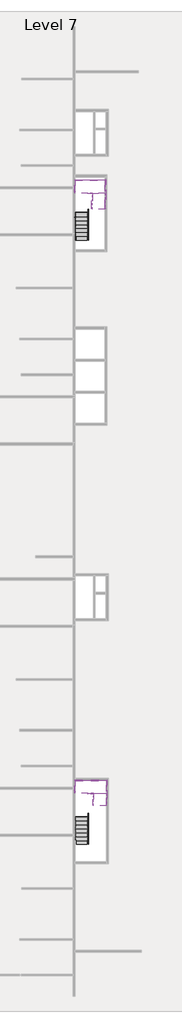
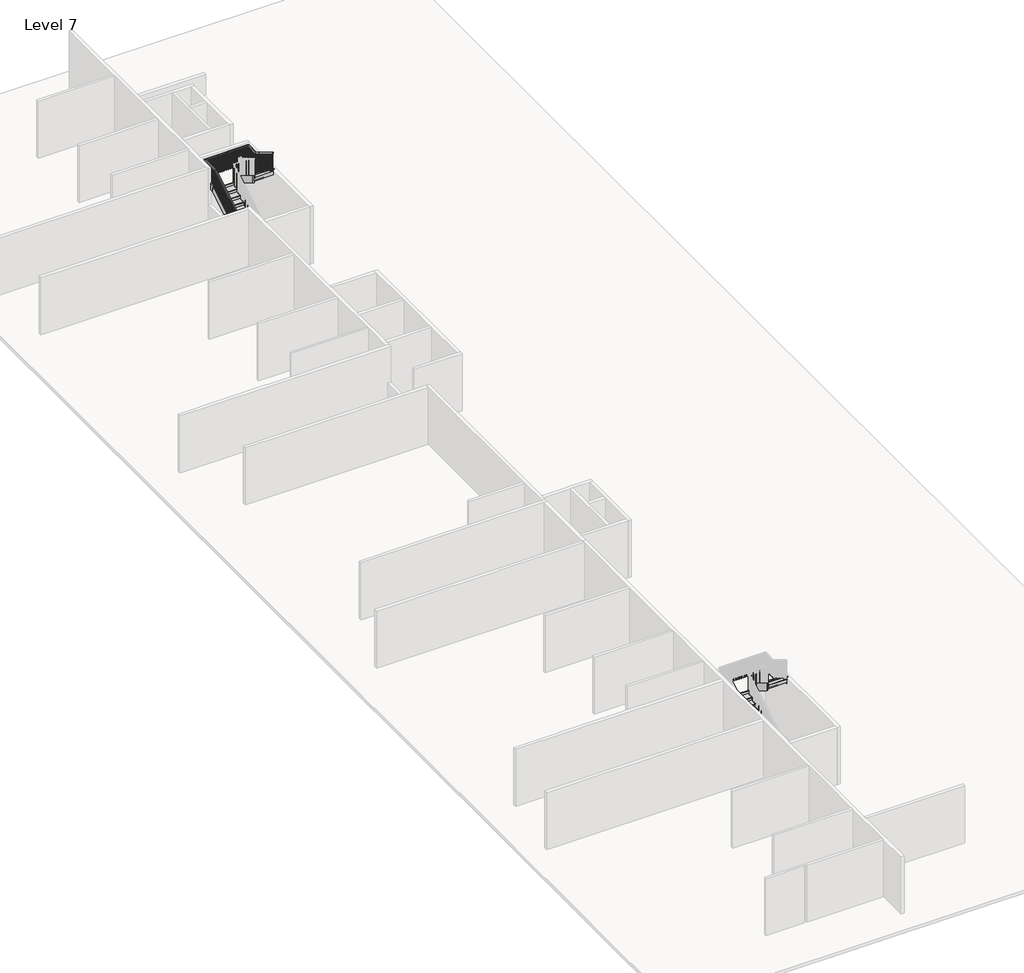
# One storey, part 8 of 8: 16 members, 4 stair flights, 2 slabs, 1 railing.
"""IFC4 building model written with IfcOpenShell, lengths in millimetres."""

from ifc_helpers import new_model, si_unit, frame, origin, place, context, project, spatial, polyline, outline, extrude, faceted_brep, transform, mapped, element, save
from components import non_monolithic_landing_71f31ac1, non_monolithic_landing_55824b8c, stair_flight_36526160, stair_flight_c8914c85, stair_flight_f72f160c, stair_flight_d5778488

model = new_model("IFC4")

# Units and contexts
model_context = context("Model", 3, world=origin())
ifc_project = project(units=[si_unit("LENGTHUNIT", "METRE", prefix="MILLI")], contexts=[model_context])

# Site, building, storey
site = spatial("IfcSite", under=ifc_project)
building = spatial("IfcBuilding", under=site)
storey = spatial("IfcBuildingStorey", under=building, Name="Level 7", Elevation=43522.6172466)

# Members
placement = place(None, origin())
element("IfcMember", 1, ObjectType="Stringer - 2\" Width", at=placement, inside=storey, context=model_context, shape_type="SweptSolid", body=[
    extrude(outline(polyline([(-23154.3851539, 43522.6172466), (-23154.3851539, 43734.7317586), (-19467.0440987, 45969.4839133), (-19381.8896422, 45664.6839133), (-22916.2996422, 43522.6172466), (-23154.3851539, 43522.6172466)])), frame((-3668.2415084, 0.0, 0.0), z_axis=(1.0, 0.0, 0.0), x_axis=(0.0, 1.0, 0.0)), (0.0, 0.0, 1.0), 50.8),
])
element("IfcMember", 2, ObjectType="Stringer - 2\" Width", at=placement, inside=storey, context=model_context, shape_type="SweptSolid", body=[
    extrude(outline(polyline([(-23154.3851539, 43522.6172466), (-23154.3851539, 43734.7317586), (-19572.9851539, 45905.2772131), (-19572.9851539, 45548.8684516), (-22916.2996422, 43522.6172466), (-23154.3851539, 43522.6172466)])), frame((-2703.0415084, 0.0, 0.0), z_axis=(1.0, 0.0, 0.0), x_axis=(0.0, 1.0, 0.0)), (0.0, 0.0, 1.0), 50.8),
])
element("IfcMember", 3, ObjectType="Stringer - 2\" Width", at=placement, inside=storey, context=model_context, shape_type="SweptSolid", body=[
    extrude(outline(polyline([(-19297.9262092, 45969.4839133), (-19383.0806657, 45664.6839133), (-20360.3851539, 46256.9896637), (-20360.3851539, 46613.3984252), (-19297.9262092, 45969.4839133)])), frame((-1382.2415084, 0.0, 0.0), z_axis=(1.0, 0.0, 0.0), x_axis=(0.0, 1.0, 0.0)), (0.0, 0.0, 1.0), 50.8),
])
element("IfcMember", 4, ObjectType="Stringer - 2\" Width", at=placement, inside=storey, context=model_context, shape_type="SweptSolid", body=[
    extrude(outline(polyline([(-19522.1851539, 46105.3984252), (-19522.1851539, 45748.9896637), (-20360.3851539, 46256.9896637), (-20360.3851539, 46613.3984252), (-19522.1851539, 46105.3984252)])), frame((-2347.4415084, 0.0, 0.0), z_axis=(1.0, 0.0, 0.0), x_axis=(0.0, 1.0, 0.0)), (0.0, 0.0, 1.0), 50.8),
])
element("IfcMember", 5, ObjectType="Stringer - 2\" Width", at=placement, inside=storey, context=model_context, shape_type="Brep", body=[
    faceted_brep([(-1382.2415084, -19297.9262092, 45969.4839133), (-1331.4415084, -19297.9262092, 45969.4839133), (-1331.4415084, -18556.9851539, 45969.4839133), (-1382.2415084, -18607.7851539, 45969.4839133), (-1382.2415084, -19383.0806657, 45664.6839133), (-1382.2415084, -18607.7851539, 45664.6839133), (-1331.4415084, -19383.0806657, 45664.6839133), (-1331.4415084, -18556.9851539, 45664.6839133)], [[[0, 1, 2, 3]], [[4, 0, 3, 5]], [[6, 4, 5, 7]], [[1, 6, 7, 2]], [[1, 0, 4, 6]], [[2, 7, 5, 3]]]),
])
element("IfcMember", 6, ObjectType="Stringer - 2\" Width", at=placement, inside=storey, context=model_context, shape_type="SweptSolid", body=[
    extrude(outline(polyline([(-1331.4415084, -18556.9851539), (-1382.2415084, -18607.7851539), (-3617.4415084, -18607.7851539), (-3668.2415084, -18556.9851539), (-1331.4415084, -18556.9851539)])), frame((0.0, 0.0, 45664.6839133), z_axis=(0.0, 0.0, 1.0), x_axis=(1.0, 0.0, 0.0)), (0.0, 0.0, 1.0), 304.8),
])
element("IfcMember", 7, ObjectType="Stringer - 2\" Width", at=placement, inside=storey, context=model_context, shape_type="Brep", body=[
    faceted_brep([(-3617.4415084, -18607.7851539, 45969.4839133), (-3668.2415084, -18556.9851539, 45969.4839133), (-3668.2415084, -19467.0440987, 45969.4839133), (-3617.4415084, -19467.0440987, 45969.4839133), (-3617.4415084, -18607.7851539, 45664.6839133), (-3617.4415084, -19381.8896422, 45664.6839133), (-3668.2415084, -18556.9851539, 45664.6839133), (-3668.2415084, -19381.8896422, 45664.6839133)], [[[0, 1, 2, 3]], [[4, 0, 3, 5]], [[6, 4, 5, 7]], [[1, 6, 7, 2]], [[1, 0, 4, 6]], [[2, 7, 5, 3]]]),
])
element("IfcMember", 8, ObjectType="Stringer - 2\" Width", at=placement, inside=storey, context=model_context, shape_type="SweptSolid", body=[
    extrude(outline(polyline([(-2703.0415084, -19572.9851539), (-2703.0415084, -19522.1851539), (-2347.4415084, -19522.1851539), (-2347.4415084, -19572.9851539), (-2703.0415084, -19572.9851539)])), frame((0.0, 0.0, 45664.6839133), z_axis=(0.0, 0.0, 1.0), x_axis=(1.0, 0.0, 0.0)), (0.0, 0.0, 1.0), 304.8),
])
element("IfcMember", 9, ObjectType="Stringer - 2\" Width", at=placement, inside=storey, context=model_context, shape_type="SweptSolid", body=[
    extrude(outline(polyline([(19841.9216096, 43522.6172466), (19841.9216096, 43734.7317586), (23249.8626649, 45800.1505799), (23335.0171214, 45495.3505799), (20080.0071214, 43522.6172466), (19841.9216096, 43522.6172466)])), frame((-3668.2415084, 0.0, 0.0), z_axis=(1.0, 0.0, 0.0), x_axis=(0.0, 1.0, 0.0)), (0.0, 0.0, 1.0), 50.8),
])
element("IfcMember", 10, ObjectType="Stringer - 2\" Width", at=placement, inside=storey, context=model_context, shape_type="SweptSolid", body=[
    extrude(outline(polyline([(19841.9216096, 43522.6172466), (19841.9216096, 43734.7317586), (23143.9216096, 45735.9438798), (23143.9216096, 45379.5351183), (20080.0071214, 43522.6172466), (19841.9216096, 43522.6172466)])), frame((-2703.0415084, 0.0, 0.0), z_axis=(1.0, 0.0, 0.0), x_axis=(0.0, 1.0, 0.0)), (0.0, 0.0, 1.0), 50.8),
])
element("IfcMember", 11, ObjectType="Stringer - 2\" Width", at=placement, inside=storey, context=model_context, shape_type="SweptSolid", body=[
    extrude(outline(polyline([(23418.9805543, 45800.1505799), (23333.8260978, 45495.3505799), (22077.1216096, 46256.9896637), (22077.1216096, 46613.3984252), (23418.9805543, 45800.1505799)])), frame((-1483.8415084, 0.0, 0.0), z_axis=(1.0, 0.0, 0.0), x_axis=(0.0, 1.0, 0.0)), (0.0, 0.0, 1.0), 50.8),
])
element("IfcMember", 12, ObjectType="Stringer - 2\" Width", at=placement, inside=storey, context=model_context, shape_type="SweptSolid", body=[
    extrude(outline(polyline([(23194.7216096, 45936.0650919), (23194.7216096, 45579.6563304), (22077.1216096, 46256.9896637), (22077.1216096, 46613.3984252), (23194.7216096, 45936.0650919)])), frame((-2449.0415084, 0.0, 0.0), z_axis=(1.0, 0.0, 0.0), x_axis=(0.0, 1.0, 0.0)), (0.0, 0.0, 1.0), 50.8),
])
element("IfcMember", 13, ObjectType="Stringer - 2\" Width", at=placement, inside=storey, context=model_context, shape_type="Brep", body=[
    faceted_brep([(-1483.8415084, 23418.9805543, 45800.1505799), (-1433.0415084, 23418.9805543, 45800.1505799), (-1433.0415084, 24159.9216096, 45800.1505799), (-1483.8415084, 24109.1216096, 45800.1505799), (-1483.8415084, 23333.8260978, 45495.3505799), (-1483.8415084, 24109.1216096, 45495.3505799), (-1433.0415084, 23333.8260978, 45495.3505799), (-1433.0415084, 24159.9216096, 45495.3505799)], [[[0, 1, 2, 3]], [[4, 0, 3, 5]], [[6, 4, 5, 7]], [[1, 6, 7, 2]], [[1, 0, 4, 6]], [[2, 7, 5, 3]]]),
])
element("IfcMember", 14, ObjectType="Stringer - 2\" Width", at=placement, inside=storey, context=model_context, shape_type="SweptSolid", body=[
    extrude(outline(polyline([(-1433.0415084, 24159.9216096), (-1483.8415084, 24109.1216096), (-3617.4415084, 24109.1216096), (-3668.2415084, 24159.9216096), (-1433.0415084, 24159.9216096)])), frame((0.0, 0.0, 45495.3505799), z_axis=(0.0, 0.0, 1.0), x_axis=(1.0, 0.0, 0.0)), (0.0, 0.0, 1.0), 304.8),
])
element("IfcMember", 15, ObjectType="Stringer - 2\" Width", at=placement, inside=storey, context=model_context, shape_type="Brep", body=[
    faceted_brep([(-3617.4415084, 24109.1216096, 45800.1505799), (-3668.2415084, 24159.9216096, 45800.1505799), (-3668.2415084, 23249.8626649, 45800.1505799), (-3617.4415084, 23249.8626649, 45800.1505799), (-3617.4415084, 24109.1216096, 45495.3505799), (-3617.4415084, 23335.0171214, 45495.3505799), (-3668.2415084, 24159.9216096, 45495.3505799), (-3668.2415084, 23335.0171214, 45495.3505799)], [[[0, 1, 2, 3]], [[4, 0, 3, 5]], [[6, 4, 5, 7]], [[1, 6, 7, 2]], [[1, 0, 4, 6]], [[2, 7, 5, 3]]]),
])
element("IfcMember", 16, ObjectType="Stringer - 2\" Width", at=placement, inside=storey, context=model_context, shape_type="SweptSolid", body=[
    extrude(outline(polyline([(-2703.0415084, 23143.9216096), (-2703.0415084, 23194.7216096), (-2449.0415084, 23194.7216096), (-2449.0415084, 23143.9216096), (-2703.0415084, 23143.9216096)])), frame((0.0, 0.0, 45495.3505799), z_axis=(0.0, 0.0, 1.0), x_axis=(1.0, 0.0, 0.0)), (0.0, 0.0, 1.0), 304.8),
])

# Railing
element("IfcRailing", 17, ObjectType="Handrail - Rectangular", at=placement, inside=storey, context=model_context, shape_type="SolidModel", body=[
    faceted_brep([(-3617.4415084, 19841.9216096, 44606.3505799), (-3617.4415084, 19841.9216096, 44546.9491197), (-3566.6415084, 19841.9216096, 44546.9491197), (-3566.6415084, 19841.9216096, 44606.3505799), (-3617.4415084, 23194.7216096, 46638.3505799), (-3617.4415084, 23208.914019, 46587.5505799), (-3566.6415084, 23208.914019, 46587.5505799), (-3566.6415084, 23194.7216096, 46638.3505799), (-3617.4415084, 24109.1216096, 46638.3505799), (-3617.4415084, 24109.1216096, 46587.5505799), (-3566.6415084, 24058.3216096, 46587.5505799), (-3566.6415084, 24058.3216096, 46638.3505799), (-1483.8415084, 24109.1216096, 46638.3505799), (-1483.8415084, 24109.1216096, 46587.5505799), (-1534.6415084, 24058.3216096, 46587.5505799), (-1534.6415084, 24058.3216096, 46638.3505799), (-1483.8415084, 23474.1216096, 46638.3505799), (-1483.8415084, 23459.9292002, 46587.5505799), (-1534.6415084, 23459.9292002, 46587.5505799), (-1534.6415084, 23474.1216096, 46638.3505799), (-1483.8415084, 23194.7216096, 46807.6839133), (-1483.8415084, 23168.3918824, 46764.2398634), (-1534.6415084, 23168.3918824, 46764.2398634), (-1534.6415084, 23194.7216096, 46807.6839133), (-1483.8415084, 22077.1216096, 47485.0172466), (-1534.6415084, 22077.1216096, 47485.0172466), (-1534.6415084, 22077.1216096, 47425.6157863), (-1483.8415084, 22077.1216096, 47425.6157863)], [[[0, 1, 2, 3]], [[1, 0, 4, 5]], [[2, 1, 5, 6]], [[3, 2, 6, 7]], [[0, 3, 7, 4]], [[5, 4, 8, 9]], [[6, 5, 9, 10]], [[7, 6, 10, 11]], [[4, 7, 11, 8]], [[9, 8, 12, 13]], [[10, 9, 13, 14]], [[11, 10, 14, 15]], [[8, 11, 15, 12]], [[13, 12, 16, 17]], [[14, 13, 17, 18]], [[15, 14, 18, 19]], [[12, 15, 19, 16]], [[17, 16, 20, 21]], [[18, 17, 21, 22]], [[19, 18, 22, 23]], [[16, 19, 23, 20]], [[24, 25, 26, 27]], [[21, 20, 24, 27]], [[22, 21, 27, 26]], [[23, 22, 26, 25]], [[20, 23, 25, 24]]]),
    extrude(outline(polyline([(22188.2466096, 47358.2673015), (22188.2466096, 46401.2839133), (22169.1966096, 46401.2839133), (22169.1966096, 47369.812756), (22188.2466096, 47358.2673015)])), frame((-1518.7665084, 0.0, 0.0), z_axis=(1.0, 0.0, 0.0), x_axis=(0.0, 1.0, 0.0)), (0.0, 0.0, 1.0), 19.05),
    extrude(outline(polyline([(22289.8466096, 47296.6915439), (22289.8466096, 46401.2839133), (22270.7966096, 46401.2839133), (22270.7966096, 47308.2369985), (22289.8466096, 47296.6915439)])), frame((-1518.7665084, 0.0, 0.0), z_axis=(1.0, 0.0, 0.0), x_axis=(0.0, 1.0, 0.0)), (0.0, 0.0, 1.0), 19.05),
    extrude(outline(polyline([(22391.4466096, 47235.1157863), (22391.4466096, 46231.9505799), (22372.3966096, 46231.9505799), (22372.3966096, 47246.6612409), (22391.4466096, 47235.1157863)])), frame((-1518.7665084, 0.0, 0.0), z_axis=(1.0, 0.0, 0.0), x_axis=(0.0, 1.0, 0.0)), (0.0, 0.0, 1.0), 19.05),
    extrude(outline(polyline([(22493.0466096, 47173.5400288), (22493.0466096, 46231.9505799), (22473.9966096, 46231.9505799), (22473.9966096, 47185.0854833), (22493.0466096, 47173.5400288)])), frame((-1518.7665084, 0.0, 0.0), z_axis=(1.0, 0.0, 0.0), x_axis=(0.0, 1.0, 0.0)), (0.0, 0.0, 1.0), 19.05),
    extrude(outline(polyline([(22594.6466096, 47111.9642712), (22594.6466096, 46231.9505799), (22575.5966096, 46231.9505799), (22575.5966096, 47123.5097257), (22594.6466096, 47111.9642712)])), frame((-1518.7665084, 0.0, 0.0), z_axis=(1.0, 0.0, 0.0), x_axis=(0.0, 1.0, 0.0)), (0.0, 0.0, 1.0), 19.05),
    extrude(outline(polyline([(22696.2466096, 47050.3885136), (22696.2466096, 46062.6172466), (22677.1966096, 46062.6172466), (22677.1966096, 47061.9339682), (22696.2466096, 47050.3885136)])), frame((-1518.7665084, 0.0, 0.0), z_axis=(1.0, 0.0, 0.0), x_axis=(0.0, 1.0, 0.0)), (0.0, 0.0, 1.0), 19.05),
    extrude(outline(polyline([(22797.8466096, 46988.812756), (22797.8466096, 46062.6172466), (22778.7966096, 46062.6172466), (22778.7966096, 47000.3582106), (22797.8466096, 46988.812756)])), frame((-1518.7665084, 0.0, 0.0), z_axis=(1.0, 0.0, 0.0), x_axis=(0.0, 1.0, 0.0)), (0.0, 0.0, 1.0), 19.05),
    extrude(outline(polyline([(22899.4466096, 46927.2369985), (22899.4466096, 46062.6172466), (22880.3966096, 46062.6172466), (22880.3966096, 46938.782453), (22899.4466096, 46927.2369985)])), frame((-1518.7665084, 0.0, 0.0), z_axis=(1.0, 0.0, 0.0), x_axis=(0.0, 1.0, 0.0)), (0.0, 0.0, 1.0), 19.05),
    extrude(outline(polyline([(23001.0466096, 46865.6612409), (23001.0466096, 45893.2839133), (22981.9966096, 45893.2839133), (22981.9966096, 46877.2066954), (23001.0466096, 46865.6612409)])), frame((-1518.7665084, 0.0, 0.0), z_axis=(1.0, 0.0, 0.0), x_axis=(0.0, 1.0, 0.0)), (0.0, 0.0, 1.0), 19.05),
    extrude(outline(polyline([(23102.6466096, 46804.0854833), (23102.6466096, 45893.2839133), (23083.5966096, 45893.2839133), (23083.5966096, 46815.6309379), (23102.6466096, 46804.0854833)])), frame((-1518.7665084, 0.0, 0.0), z_axis=(1.0, 0.0, 0.0), x_axis=(0.0, 1.0, 0.0)), (0.0, 0.0, 1.0), 19.05),
    extrude(outline(polyline([(23280.4466096, 46696.3279076), (23280.4466096, 45723.9505799), (23261.3966096, 45723.9505799), (23261.3966096, 46707.8733621), (23280.4466096, 46696.3279076)])), frame((-1518.7665084, 0.0, 0.0), z_axis=(1.0, 0.0, 0.0), x_axis=(0.0, 1.0, 0.0)), (0.0, 0.0, 1.0), 19.05),
    extrude(outline(polyline([(23382.0466096, 46634.75215), (23382.0466096, 45723.9505799), (23362.9966096, 45723.9505799), (23362.9966096, 46646.2976045), (23382.0466096, 46634.75215)])), frame((-1518.7665084, 0.0, 0.0), z_axis=(1.0, 0.0, 0.0), x_axis=(0.0, 1.0, 0.0)), (0.0, 0.0, 1.0), 19.05),
    extrude(outline(polyline([(-1499.7165084, 23483.6466096), (-1499.7165084, 23464.5966096), (-1518.7665084, 23464.5966096), (-1518.7665084, 23483.6466096), (-1499.7165084, 23483.6466096)])), frame((0.0, 0.0, 45723.9505799), z_axis=(0.0, 0.0, 1.0), x_axis=(1.0, 0.0, 0.0)), (0.0, 0.0, 1.0), 863.6),
    extrude(outline(polyline([(-1499.7165084, 23585.2466096), (-1499.7165084, 23566.1966096), (-1518.7665084, 23566.1966096), (-1518.7665084, 23585.2466096), (-1499.7165084, 23585.2466096)])), frame((0.0, 0.0, 45723.9505799), z_axis=(0.0, 0.0, 1.0), x_axis=(1.0, 0.0, 0.0)), (0.0, 0.0, 1.0), 863.6),
    extrude(outline(polyline([(-1499.7165084, 23686.8466096), (-1499.7165084, 23667.7966096), (-1518.7665084, 23667.7966096), (-1518.7665084, 23686.8466096), (-1499.7165084, 23686.8466096)])), frame((0.0, 0.0, 45723.9505799), z_axis=(0.0, 0.0, 1.0), x_axis=(1.0, 0.0, 0.0)), (0.0, 0.0, 1.0), 863.6),
    extrude(outline(polyline([(-1499.7165084, 23788.4466096), (-1499.7165084, 23769.3966096), (-1518.7665084, 23769.3966096), (-1518.7665084, 23788.4466096), (-1499.7165084, 23788.4466096)])), frame((0.0, 0.0, 45723.9505799), z_axis=(0.0, 0.0, 1.0), x_axis=(1.0, 0.0, 0.0)), (0.0, 0.0, 1.0), 863.6),
    extrude(outline(polyline([(-1499.7165084, 23890.0466096), (-1499.7165084, 23870.9966096), (-1518.7665084, 23870.9966096), (-1518.7665084, 23890.0466096), (-1499.7165084, 23890.0466096)])), frame((0.0, 0.0, 45723.9505799), z_axis=(0.0, 0.0, 1.0), x_axis=(1.0, 0.0, 0.0)), (0.0, 0.0, 1.0), 863.6),
    extrude(outline(polyline([(-1499.7165084, 23991.6466096), (-1499.7165084, 23972.5966096), (-1518.7665084, 23972.5966096), (-1518.7665084, 23991.6466096), (-1499.7165084, 23991.6466096)])), frame((0.0, 0.0, 45723.9505799), z_axis=(0.0, 0.0, 1.0), x_axis=(1.0, 0.0, 0.0)), (0.0, 0.0, 1.0), 863.6),
    extrude(outline(polyline([(-1569.5665084, 24093.2466096), (-1550.5165084, 24093.2466096), (-1550.5165084, 24074.1966096), (-1569.5665084, 24074.1966096), (-1569.5665084, 24093.2466096)])), frame((0.0, 0.0, 45723.9505799), z_axis=(0.0, 0.0, 1.0), x_axis=(1.0, 0.0, 0.0)), (0.0, 0.0, 1.0), 863.6),
    extrude(outline(polyline([(-1671.1665084, 24093.2466096), (-1652.1165084, 24093.2466096), (-1652.1165084, 24074.1966096), (-1671.1665084, 24074.1966096), (-1671.1665084, 24093.2466096)])), frame((0.0, 0.0, 45723.9505799), z_axis=(0.0, 0.0, 1.0), x_axis=(1.0, 0.0, 0.0)), (0.0, 0.0, 1.0), 863.6),
    extrude(outline(polyline([(-1772.7665084, 24093.2466096), (-1753.7165084, 24093.2466096), (-1753.7165084, 24074.1966096), (-1772.7665084, 24074.1966096), (-1772.7665084, 24093.2466096)])), frame((0.0, 0.0, 45723.9505799), z_axis=(0.0, 0.0, 1.0), x_axis=(1.0, 0.0, 0.0)), (0.0, 0.0, 1.0), 863.6),
    extrude(outline(polyline([(-1874.3665084, 24093.2466096), (-1855.3165084, 24093.2466096), (-1855.3165084, 24074.1966096), (-1874.3665084, 24074.1966096), (-1874.3665084, 24093.2466096)])), frame((0.0, 0.0, 45723.9505799), z_axis=(0.0, 0.0, 1.0), x_axis=(1.0, 0.0, 0.0)), (0.0, 0.0, 1.0), 863.6),
    extrude(outline(polyline([(-1975.9665084, 24093.2466096), (-1956.9165084, 24093.2466096), (-1956.9165084, 24074.1966096), (-1975.9665084, 24074.1966096), (-1975.9665084, 24093.2466096)])), frame((0.0, 0.0, 45723.9505799), z_axis=(0.0, 0.0, 1.0), x_axis=(1.0, 0.0, 0.0)), (0.0, 0.0, 1.0), 863.6),
    extrude(outline(polyline([(-2077.5665084, 24093.2466096), (-2058.5165084, 24093.2466096), (-2058.5165084, 24074.1966096), (-2077.5665084, 24074.1966096), (-2077.5665084, 24093.2466096)])), frame((0.0, 0.0, 45723.9505799), z_axis=(0.0, 0.0, 1.0), x_axis=(1.0, 0.0, 0.0)), (0.0, 0.0, 1.0), 863.6),
    extrude(outline(polyline([(-2179.1665084, 24093.2466096), (-2160.1165084, 24093.2466096), (-2160.1165084, 24074.1966096), (-2179.1665084, 24074.1966096), (-2179.1665084, 24093.2466096)])), frame((0.0, 0.0, 45723.9505799), z_axis=(0.0, 0.0, 1.0), x_axis=(1.0, 0.0, 0.0)), (0.0, 0.0, 1.0), 863.6),
    extrude(outline(polyline([(-2280.7665084, 24093.2466096), (-2261.7165084, 24093.2466096), (-2261.7165084, 24074.1966096), (-2280.7665084, 24074.1966096), (-2280.7665084, 24093.2466096)])), frame((0.0, 0.0, 45723.9505799), z_axis=(0.0, 0.0, 1.0), x_axis=(1.0, 0.0, 0.0)), (0.0, 0.0, 1.0), 863.6),
    extrude(outline(polyline([(-2382.3665084, 24093.2466096), (-2363.3165084, 24093.2466096), (-2363.3165084, 24074.1966096), (-2382.3665084, 24074.1966096), (-2382.3665084, 24093.2466096)])), frame((0.0, 0.0, 45723.9505799), z_axis=(0.0, 0.0, 1.0), x_axis=(1.0, 0.0, 0.0)), (0.0, 0.0, 1.0), 863.6),
    extrude(outline(polyline([(-2483.9665084, 24093.2466096), (-2464.9165084, 24093.2466096), (-2464.9165084, 24074.1966096), (-2483.9665084, 24074.1966096), (-2483.9665084, 24093.2466096)])), frame((0.0, 0.0, 45723.9505799), z_axis=(0.0, 0.0, 1.0), x_axis=(1.0, 0.0, 0.0)), (0.0, 0.0, 1.0), 863.6),
    extrude(outline(polyline([(-2585.5665084, 24093.2466096), (-2566.5165084, 24093.2466096), (-2566.5165084, 24074.1966096), (-2585.5665084, 24074.1966096), (-2585.5665084, 24093.2466096)])), frame((0.0, 0.0, 45723.9505799), z_axis=(0.0, 0.0, 1.0), x_axis=(1.0, 0.0, 0.0)), (0.0, 0.0, 1.0), 863.6),
    extrude(outline(polyline([(-2687.1665084, 24093.2466096), (-2668.1165084, 24093.2466096), (-2668.1165084, 24074.1966096), (-2687.1665084, 24074.1966096), (-2687.1665084, 24093.2466096)])), frame((0.0, 0.0, 45723.9505799), z_axis=(0.0, 0.0, 1.0), x_axis=(1.0, 0.0, 0.0)), (0.0, 0.0, 1.0), 863.6),
    extrude(outline(polyline([(-2788.7665084, 24093.2466096), (-2769.7165084, 24093.2466096), (-2769.7165084, 24074.1966096), (-2788.7665084, 24074.1966096), (-2788.7665084, 24093.2466096)])), frame((0.0, 0.0, 45723.9505799), z_axis=(0.0, 0.0, 1.0), x_axis=(1.0, 0.0, 0.0)), (0.0, 0.0, 1.0), 863.6),
    extrude(outline(polyline([(-2890.3665084, 24093.2466096), (-2871.3165084, 24093.2466096), (-2871.3165084, 24074.1966096), (-2890.3665084, 24074.1966096), (-2890.3665084, 24093.2466096)])), frame((0.0, 0.0, 45723.9505799), z_axis=(0.0, 0.0, 1.0), x_axis=(1.0, 0.0, 0.0)), (0.0, 0.0, 1.0), 863.6),
    extrude(outline(polyline([(-2991.9665084, 24093.2466096), (-2972.9165084, 24093.2466096), (-2972.9165084, 24074.1966096), (-2991.9665084, 24074.1966096), (-2991.9665084, 24093.2466096)])), frame((0.0, 0.0, 45723.9505799), z_axis=(0.0, 0.0, 1.0), x_axis=(1.0, 0.0, 0.0)), (0.0, 0.0, 1.0), 863.6),
    extrude(outline(polyline([(-3093.5665084, 24093.2466096), (-3074.5165084, 24093.2466096), (-3074.5165084, 24074.1966096), (-3093.5665084, 24074.1966096), (-3093.5665084, 24093.2466096)])), frame((0.0, 0.0, 45723.9505799), z_axis=(0.0, 0.0, 1.0), x_axis=(1.0, 0.0, 0.0)), (0.0, 0.0, 1.0), 863.6),
    extrude(outline(polyline([(-3195.1665084, 24093.2466096), (-3176.1165084, 24093.2466096), (-3176.1165084, 24074.1966096), (-3195.1665084, 24074.1966096), (-3195.1665084, 24093.2466096)])), frame((0.0, 0.0, 45723.9505799), z_axis=(0.0, 0.0, 1.0), x_axis=(1.0, 0.0, 0.0)), (0.0, 0.0, 1.0), 863.6),
    extrude(outline(polyline([(-3296.7665084, 24093.2466096), (-3277.7165084, 24093.2466096), (-3277.7165084, 24074.1966096), (-3296.7665084, 24074.1966096), (-3296.7665084, 24093.2466096)])), frame((0.0, 0.0, 45723.9505799), z_axis=(0.0, 0.0, 1.0), x_axis=(1.0, 0.0, 0.0)), (0.0, 0.0, 1.0), 863.6),
    extrude(outline(polyline([(-3398.3665084, 24093.2466096), (-3379.3165084, 24093.2466096), (-3379.3165084, 24074.1966096), (-3398.3665084, 24074.1966096), (-3398.3665084, 24093.2466096)])), frame((0.0, 0.0, 45723.9505799), z_axis=(0.0, 0.0, 1.0), x_axis=(1.0, 0.0, 0.0)), (0.0, 0.0, 1.0), 863.6),
    extrude(outline(polyline([(-3499.9665084, 24093.2466096), (-3480.9165084, 24093.2466096), (-3480.9165084, 24074.1966096), (-3499.9665084, 24074.1966096), (-3499.9665084, 24093.2466096)])), frame((0.0, 0.0, 45723.9505799), z_axis=(0.0, 0.0, 1.0), x_axis=(1.0, 0.0, 0.0)), (0.0, 0.0, 1.0), 863.6),
    extrude(outline(polyline([(-3601.5665084, 23997.9966096), (-3601.5665084, 24017.0466096), (-3582.5165084, 24017.0466096), (-3582.5165084, 23997.9966096), (-3601.5665084, 23997.9966096)])), frame((0.0, 0.0, 45723.9505799), z_axis=(0.0, 0.0, 1.0), x_axis=(1.0, 0.0, 0.0)), (0.0, 0.0, 1.0), 863.6),
    extrude(outline(polyline([(-3601.5665084, 23896.3966096), (-3601.5665084, 23915.4466096), (-3582.5165084, 23915.4466096), (-3582.5165084, 23896.3966096), (-3601.5665084, 23896.3966096)])), frame((0.0, 0.0, 45723.9505799), z_axis=(0.0, 0.0, 1.0), x_axis=(1.0, 0.0, 0.0)), (0.0, 0.0, 1.0), 863.6),
    extrude(outline(polyline([(-3601.5665084, 23794.7966096), (-3601.5665084, 23813.8466096), (-3582.5165084, 23813.8466096), (-3582.5165084, 23794.7966096), (-3601.5665084, 23794.7966096)])), frame((0.0, 0.0, 45723.9505799), z_axis=(0.0, 0.0, 1.0), x_axis=(1.0, 0.0, 0.0)), (0.0, 0.0, 1.0), 863.6),
    extrude(outline(polyline([(-3601.5665084, 23693.1966096), (-3601.5665084, 23712.2466096), (-3582.5165084, 23712.2466096), (-3582.5165084, 23693.1966096), (-3601.5665084, 23693.1966096)])), frame((0.0, 0.0, 45723.9505799), z_axis=(0.0, 0.0, 1.0), x_axis=(1.0, 0.0, 0.0)), (0.0, 0.0, 1.0), 863.6),
    extrude(outline(polyline([(-3601.5665084, 23591.5966096), (-3601.5665084, 23610.6466096), (-3582.5165084, 23610.6466096), (-3582.5165084, 23591.5966096), (-3601.5665084, 23591.5966096)])), frame((0.0, 0.0, 45723.9505799), z_axis=(0.0, 0.0, 1.0), x_axis=(1.0, 0.0, 0.0)), (0.0, 0.0, 1.0), 863.6),
    extrude(outline(polyline([(-3601.5665084, 23489.9966096), (-3601.5665084, 23509.0466096), (-3582.5165084, 23509.0466096), (-3582.5165084, 23489.9966096), (-3601.5665084, 23489.9966096)])), frame((0.0, 0.0, 45723.9505799), z_axis=(0.0, 0.0, 1.0), x_axis=(1.0, 0.0, 0.0)), (0.0, 0.0, 1.0), 863.6),
    extrude(outline(polyline([(-3601.5665084, 23388.3966096), (-3601.5665084, 23407.4466096), (-3582.5165084, 23407.4466096), (-3582.5165084, 23388.3966096), (-3601.5665084, 23388.3966096)])), frame((0.0, 0.0, 45723.9505799), z_axis=(0.0, 0.0, 1.0), x_axis=(1.0, 0.0, 0.0)), (0.0, 0.0, 1.0), 863.6),
    extrude(outline(polyline([(-3601.5665084, 23286.7966096), (-3601.5665084, 23305.8466096), (-3582.5165084, 23305.8466096), (-3582.5165084, 23286.7966096), (-3601.5665084, 23286.7966096)])), frame((0.0, 0.0, 45723.9505799), z_axis=(0.0, 0.0, 1.0), x_axis=(1.0, 0.0, 0.0)), (0.0, 0.0, 1.0), 863.6),
    extrude(outline(polyline([(23102.6466096, 46523.1460894), (23102.6466096, 45554.6172466), (23083.5966096, 45554.6172466), (23083.5966096, 46511.6006348), (23102.6466096, 46523.1460894)])), frame((-3601.5665084, 0.0, 0.0), z_axis=(1.0, 0.0, 0.0), x_axis=(0.0, 1.0, 0.0)), (0.0, 0.0, 1.0), 19.05),
    extrude(outline(polyline([(23001.0466096, 46461.5703318), (23001.0466096, 45554.6172466), (22981.9966096, 45554.6172466), (22981.9966096, 46450.0248773), (23001.0466096, 46461.5703318)])), frame((-3601.5665084, 0.0, 0.0), z_axis=(1.0, 0.0, 0.0), x_axis=(0.0, 1.0, 0.0)), (0.0, 0.0, 1.0), 19.05),
    extrude(outline(polyline([(22899.4466096, 46399.9945742), (22899.4466096, 45385.2839133), (22880.3966096, 45385.2839133), (22880.3966096, 46388.4491197), (22899.4466096, 46399.9945742)])), frame((-3601.5665084, 0.0, 0.0), z_axis=(1.0, 0.0, 0.0), x_axis=(0.0, 1.0, 0.0)), (0.0, 0.0, 1.0), 19.05),
    extrude(outline(polyline([(22797.8466096, 46338.4188166), (22797.8466096, 45385.2839133), (22778.7966096, 45385.2839133), (22778.7966096, 46326.8733621), (22797.8466096, 46338.4188166)])), frame((-3601.5665084, 0.0, 0.0), z_axis=(1.0, 0.0, 0.0), x_axis=(0.0, 1.0, 0.0)), (0.0, 0.0, 1.0), 19.05),
    extrude(outline(polyline([(22696.2466096, 46276.8430591), (22696.2466096, 45385.2839133), (22677.1966096, 45385.2839133), (22677.1966096, 46265.2976045), (22696.2466096, 46276.8430591)])), frame((-3601.5665084, 0.0, 0.0), z_axis=(1.0, 0.0, 0.0), x_axis=(0.0, 1.0, 0.0)), (0.0, 0.0, 1.0), 19.05),
    extrude(outline(polyline([(22594.6466096, 46215.2673015), (22594.6466096, 45215.9505799), (22575.5966096, 45215.9505799), (22575.5966096, 46203.721847), (22594.6466096, 46215.2673015)])), frame((-3601.5665084, 0.0, 0.0), z_axis=(1.0, 0.0, 0.0), x_axis=(0.0, 1.0, 0.0)), (0.0, 0.0, 1.0), 19.05),
    extrude(outline(polyline([(22493.0466096, 46153.6915439), (22493.0466096, 45215.9505799), (22473.9966096, 45215.9505799), (22473.9966096, 46142.1460894), (22493.0466096, 46153.6915439)])), frame((-3601.5665084, 0.0, 0.0), z_axis=(1.0, 0.0, 0.0), x_axis=(0.0, 1.0, 0.0)), (0.0, 0.0, 1.0), 19.05),
    extrude(outline(polyline([(22391.4466096, 46092.1157863), (22391.4466096, 45215.9505799), (22372.3966096, 45215.9505799), (22372.3966096, 46080.5703318), (22391.4466096, 46092.1157863)])), frame((-3601.5665084, 0.0, 0.0), z_axis=(1.0, 0.0, 0.0), x_axis=(0.0, 1.0, 0.0)), (0.0, 0.0, 1.0), 19.05),
    extrude(outline(polyline([(22289.8466096, 46030.5400288), (22289.8466096, 45046.6172466), (22270.7966096, 45046.6172466), (22270.7966096, 46018.9945742), (22289.8466096, 46030.5400288)])), frame((-3601.5665084, 0.0, 0.0), z_axis=(1.0, 0.0, 0.0), x_axis=(0.0, 1.0, 0.0)), (0.0, 0.0, 1.0), 19.05),
    extrude(outline(polyline([(22188.2466096, 45968.9642712), (22188.2466096, 45046.6172466), (22169.1966096, 45046.6172466), (22169.1966096, 45957.4188166), (22188.2466096, 45968.9642712)])), frame((-3601.5665084, 0.0, 0.0), z_axis=(1.0, 0.0, 0.0), x_axis=(0.0, 1.0, 0.0)), (0.0, 0.0, 1.0), 19.05),
    extrude(outline(polyline([(22086.6466096, 45907.3885136), (22086.6466096, 45046.6172466), (22067.5966096, 45046.6172466), (22067.5966096, 45895.8430591), (22086.6466096, 45907.3885136)])), frame((-3601.5665084, 0.0, 0.0), z_axis=(1.0, 0.0, 0.0), x_axis=(0.0, 1.0, 0.0)), (0.0, 0.0, 1.0), 19.05),
    extrude(outline(polyline([(21985.0466096, 45845.812756), (21985.0466096, 44877.2839133), (21965.9966096, 44877.2839133), (21965.9966096, 45834.2673015), (21985.0466096, 45845.812756)])), frame((-3601.5665084, 0.0, 0.0), z_axis=(1.0, 0.0, 0.0), x_axis=(0.0, 1.0, 0.0)), (0.0, 0.0, 1.0), 19.05),
    extrude(outline(polyline([(21883.4466096, 45784.2369985), (21883.4466096, 44877.2839133), (21864.3966096, 44877.2839133), (21864.3966096, 45772.6915439), (21883.4466096, 45784.2369985)])), frame((-3601.5665084, 0.0, 0.0), z_axis=(1.0, 0.0, 0.0), x_axis=(0.0, 1.0, 0.0)), (0.0, 0.0, 1.0), 19.05),
    extrude(outline(polyline([(21781.8466096, 45722.6612409), (21781.8466096, 44707.9505799), (21762.7966096, 44707.9505799), (21762.7966096, 45711.1157863), (21781.8466096, 45722.6612409)])), frame((-3601.5665084, 0.0, 0.0), z_axis=(1.0, 0.0, 0.0), x_axis=(0.0, 1.0, 0.0)), (0.0, 0.0, 1.0), 19.05),
    extrude(outline(polyline([(21680.2466096, 45661.0854833), (21680.2466096, 44707.9505799), (21661.1966096, 44707.9505799), (21661.1966096, 45649.5400288), (21680.2466096, 45661.0854833)])), frame((-3601.5665084, 0.0, 0.0), z_axis=(1.0, 0.0, 0.0), x_axis=(0.0, 1.0, 0.0)), (0.0, 0.0, 1.0), 19.05),
    extrude(outline(polyline([(21578.6466096, 45599.5097257), (21578.6466096, 44707.9505799), (21559.5966096, 44707.9505799), (21559.5966096, 45587.9642712), (21578.6466096, 45599.5097257)])), frame((-3601.5665084, 0.0, 0.0), z_axis=(1.0, 0.0, 0.0), x_axis=(0.0, 1.0, 0.0)), (0.0, 0.0, 1.0), 19.05),
    extrude(outline(polyline([(21477.0466096, 45537.9339682), (21477.0466096, 44538.6172466), (21457.9966096, 44538.6172466), (21457.9966096, 45526.3885136), (21477.0466096, 45537.9339682)])), frame((-3601.5665084, 0.0, 0.0), z_axis=(1.0, 0.0, 0.0), x_axis=(0.0, 1.0, 0.0)), (0.0, 0.0, 1.0), 19.05),
    extrude(outline(polyline([(21375.4466096, 45476.3582106), (21375.4466096, 44538.6172466), (21356.3966096, 44538.6172466), (21356.3966096, 45464.812756), (21375.4466096, 45476.3582106)])), frame((-3601.5665084, 0.0, 0.0), z_axis=(1.0, 0.0, 0.0), x_axis=(0.0, 1.0, 0.0)), (0.0, 0.0, 1.0), 19.05),
    extrude(outline(polyline([(21273.8466096, 45414.782453), (21273.8466096, 44538.6172466), (21254.7966096, 44538.6172466), (21254.7966096, 45403.2369985), (21273.8466096, 45414.782453)])), frame((-3601.5665084, 0.0, 0.0), z_axis=(1.0, 0.0, 0.0), x_axis=(0.0, 1.0, 0.0)), (0.0, 0.0, 1.0), 19.05),
    extrude(outline(polyline([(21172.2466096, 45353.2066954), (21172.2466096, 44369.2839133), (21153.1966096, 44369.2839133), (21153.1966096, 45341.6612409), (21172.2466096, 45353.2066954)])), frame((-3601.5665084, 0.0, 0.0), z_axis=(1.0, 0.0, 0.0), x_axis=(0.0, 1.0, 0.0)), (0.0, 0.0, 1.0), 19.05),
    extrude(outline(polyline([(21070.6466096, 45291.6309379), (21070.6466096, 44369.2839133), (21051.5966096, 44369.2839133), (21051.5966096, 45280.0854833), (21070.6466096, 45291.6309379)])), frame((-3601.5665084, 0.0, 0.0), z_axis=(1.0, 0.0, 0.0), x_axis=(0.0, 1.0, 0.0)), (0.0, 0.0, 1.0), 19.05),
    extrude(outline(polyline([(20969.0466096, 45230.0551803), (20969.0466096, 44369.2839133), (20949.9966096, 44369.2839133), (20949.9966096, 45218.5097257), (20969.0466096, 45230.0551803)])), frame((-3601.5665084, 0.0, 0.0), z_axis=(1.0, 0.0, 0.0), x_axis=(0.0, 1.0, 0.0)), (0.0, 0.0, 1.0), 19.05),
    extrude(outline(polyline([(20867.4466096, 45168.4794227), (20867.4466096, 44199.9505799), (20848.3966096, 44199.9505799), (20848.3966096, 45156.9339682), (20867.4466096, 45168.4794227)])), frame((-3601.5665084, 0.0, 0.0), z_axis=(1.0, 0.0, 0.0), x_axis=(0.0, 1.0, 0.0)), (0.0, 0.0, 1.0), 19.05),
    extrude(outline(polyline([(20765.8466096, 45106.9036651), (20765.8466096, 44199.9505799), (20746.7966096, 44199.9505799), (20746.7966096, 45095.3582106), (20765.8466096, 45106.9036651)])), frame((-3601.5665084, 0.0, 0.0), z_axis=(1.0, 0.0, 0.0), x_axis=(0.0, 1.0, 0.0)), (0.0, 0.0, 1.0), 19.05),
    extrude(outline(polyline([(20664.2466096, 45045.3279076), (20664.2466096, 44030.6172466), (20645.1966096, 44030.6172466), (20645.1966096, 45033.782453), (20664.2466096, 45045.3279076)])), frame((-3601.5665084, 0.0, 0.0), z_axis=(1.0, 0.0, 0.0), x_axis=(0.0, 1.0, 0.0)), (0.0, 0.0, 1.0), 19.05),
    extrude(outline(polyline([(20562.6466096, 44983.75215), (20562.6466096, 44030.6172466), (20543.5966096, 44030.6172466), (20543.5966096, 44972.2066954), (20562.6466096, 44983.75215)])), frame((-3601.5665084, 0.0, 0.0), z_axis=(1.0, 0.0, 0.0), x_axis=(0.0, 1.0, 0.0)), (0.0, 0.0, 1.0), 19.05),
    extrude(outline(polyline([(20461.0466096, 44922.1763924), (20461.0466096, 44030.6172466), (20441.9966096, 44030.6172466), (20441.9966096, 44910.6309379), (20461.0466096, 44922.1763924)])), frame((-3601.5665084, 0.0, 0.0), z_axis=(1.0, 0.0, 0.0), x_axis=(0.0, 1.0, 0.0)), (0.0, 0.0, 1.0), 19.05),
    extrude(outline(polyline([(20359.4466096, 44860.6006348), (20359.4466096, 43861.2839133), (20340.3966096, 43861.2839133), (20340.3966096, 44849.0551803), (20359.4466096, 44860.6006348)])), frame((-3601.5665084, 0.0, 0.0), z_axis=(1.0, 0.0, 0.0), x_axis=(0.0, 1.0, 0.0)), (0.0, 0.0, 1.0), 19.05),
    extrude(outline(polyline([(20257.8466096, 44799.0248773), (20257.8466096, 43861.2839133), (20238.7966096, 43861.2839133), (20238.7966096, 44787.4794227), (20257.8466096, 44799.0248773)])), frame((-3601.5665084, 0.0, 0.0), z_axis=(1.0, 0.0, 0.0), x_axis=(0.0, 1.0, 0.0)), (0.0, 0.0, 1.0), 19.05),
    extrude(outline(polyline([(20156.2466096, 44737.4491197), (20156.2466096, 43861.2839133), (20137.1966096, 43861.2839133), (20137.1966096, 44725.9036651), (20156.2466096, 44737.4491197)])), frame((-3601.5665084, 0.0, 0.0), z_axis=(1.0, 0.0, 0.0), x_axis=(0.0, 1.0, 0.0)), (0.0, 0.0, 1.0), 19.05),
    extrude(outline(polyline([(20054.6466096, 44675.8733621), (20054.6466096, 43691.9505799), (20035.5966096, 43691.9505799), (20035.5966096, 44664.3279076), (20054.6466096, 44675.8733621)])), frame((-3601.5665084, 0.0, 0.0), z_axis=(1.0, 0.0, 0.0), x_axis=(0.0, 1.0, 0.0)), (0.0, 0.0, 1.0), 19.05),
    extrude(outline(polyline([(19953.0466096, 44614.2976045), (19953.0466096, 43691.9505799), (19933.9966096, 43691.9505799), (19933.9966096, 44602.75215), (19953.0466096, 44614.2976045)])), frame((-3601.5665084, 0.0, 0.0), z_axis=(1.0, 0.0, 0.0), x_axis=(0.0, 1.0, 0.0)), (0.0, 0.0, 1.0), 19.05),
    extrude(outline(polyline([(23204.2466096, 46742.5097257), (23204.2466096, 45723.9505799), (23185.1966096, 45723.9505799), (23185.1966096, 46754.0551803), (23204.2466096, 46742.5097257)])), frame((-1518.7665084, 0.0, 0.0), z_axis=(1.0, 0.0, 0.0), x_axis=(0.0, 1.0, 0.0)), (0.0, 0.0, 1.0), 19.05),
    extrude(outline(polyline([(-1518.7665084, 24093.2466096), (-1499.7165084, 24093.2466096), (-1499.7165084, 24074.1966096), (-1518.7665084, 24074.1966096), (-1518.7665084, 24093.2466096)])), frame((0.0, 0.0, 45723.9505799), z_axis=(0.0, 0.0, 1.0), x_axis=(1.0, 0.0, 0.0)), (0.0, 0.0, 1.0), 863.6),
    extrude(outline(polyline([(-3601.5665084, 24074.1966096), (-3601.5665084, 24093.2466096), (-3582.5165084, 24093.2466096), (-3582.5165084, 24074.1966096), (-3601.5665084, 24074.1966096)])), frame((0.0, 0.0, 45723.9505799), z_axis=(0.0, 0.0, 1.0), x_axis=(1.0, 0.0, 0.0)), (0.0, 0.0, 1.0), 863.6),
    extrude(outline(polyline([(23204.2466096, 46584.721847), (23204.2466096, 45723.9505799), (23185.1966096, 45723.9505799), (23185.1966096, 46573.1763924), (23204.2466096, 46584.721847)])), frame((-3601.5665084, 0.0, 0.0), z_axis=(1.0, 0.0, 0.0), x_axis=(0.0, 1.0, 0.0)), (0.0, 0.0, 1.0), 19.05),
    extrude(outline(polyline([(22096.1716096, 47414.0703318), (22096.1716096, 46401.2839133), (22077.1216096, 46401.2839133), (22077.1216096, 47425.6157863), (22096.1716096, 47414.0703318)])), frame((-1518.7665084, 0.0, 0.0), z_axis=(1.0, 0.0, 0.0), x_axis=(0.0, 1.0, 0.0)), (0.0, 0.0, 1.0), 19.05),
    extrude(outline(polyline([(19860.9716096, 44558.4945742), (19860.9716096, 43691.9505799), (19841.9216096, 43691.9505799), (19841.9216096, 44546.9491197), (19860.9716096, 44558.4945742)])), frame((-3601.5665084, 0.0, 0.0), z_axis=(1.0, 0.0, 0.0), x_axis=(0.0, 1.0, 0.0)), (0.0, 0.0, 1.0), 19.05),
])

# Slabs
non_monolithic_landing_shape = non_monolithic_landing_71f31ac1(model_context)
element("IfcSlab", 18, ObjectType="Non-Monolithic Landing", at=placement, inside=storey, context=model_context, shape_type="MappedRepresentation", body=[
    mapped(non_monolithic_landing_shape, transform((0.0, 0.0, 0.0), x_axis=(1.0, 0.0, 0.0), y_axis=(0.0, 1.0, 0.0), z_axis=(0.0, 0.0, 1.0))),
])
non_monolithic_landing_2_shape = non_monolithic_landing_55824b8c(model_context)
element("IfcSlab", 19, ObjectType="Non-Monolithic Landing", at=placement, inside=storey, context=model_context, shape_type="MappedRepresentation", body=[
    mapped(non_monolithic_landing_2_shape, transform((0.0, 0.0, 0.0), x_axis=(1.0, 0.0, 0.0), y_axis=(0.0, 1.0, 0.0), z_axis=(0.0, 0.0, 1.0))),
])

# Stair flights
stair_flight_shape = stair_flight_36526160(model_context)
element("IfcStairFlight", 20, ObjectType="2\" Tread 1\" Nosing 1/4\" Riser", at=placement, inside=storey, context=model_context, shape_type="MappedRepresentation", body=[
    mapped(stair_flight_shape, transform((0.0, 0.0, 0.0), x_axis=(1.0, 0.0, 0.0), y_axis=(0.0, 1.0, 0.0), z_axis=(0.0, 0.0, 1.0))),
])
stair_flight_2_shape = stair_flight_c8914c85(model_context)
element("IfcStairFlight", 21, ObjectType="2\" Tread 1\" Nosing 1/4\" Riser", at=placement, inside=storey, context=model_context, shape_type="MappedRepresentation", body=[
    mapped(stair_flight_2_shape, transform((0.0, 0.0, 0.0), x_axis=(1.0, 0.0, 0.0), y_axis=(0.0, 1.0, 0.0), z_axis=(0.0, 0.0, 1.0))),
])
stair_flight_3_shape = stair_flight_f72f160c(model_context)
element("IfcStairFlight", 22, ObjectType="2\" Tread 1\" Nosing 1/4\" Riser", at=placement, inside=storey, context=model_context, shape_type="MappedRepresentation", body=[
    mapped(stair_flight_3_shape, transform((0.0, 0.0, 0.0), x_axis=(1.0, 0.0, 0.0), y_axis=(0.0, 1.0, 0.0), z_axis=(0.0, 0.0, 1.0))),
])
stair_flight_4_shape = stair_flight_d5778488(model_context)
element("IfcStairFlight", 23, ObjectType="2\" Tread 1\" Nosing 1/4\" Riser", at=placement, inside=storey, context=model_context, shape_type="MappedRepresentation", body=[
    mapped(stair_flight_4_shape, transform((0.0, 0.0, 0.0), x_axis=(1.0, 0.0, 0.0), y_axis=(0.0, 1.0, 0.0), z_axis=(0.0, 0.0, 1.0))),
])

save(model, "model.ifc")

# Revit data of these elements
# Type "Handrail - Rectangular"
#   Assembly Code = "C2010400"
#   built-in parameter 1008612 = 0.0416667 (stored number, unit not read)
#   built-in parameter 1008611 = 0.0416667 (stored number, unit not read)
#   built-in parameter 1008609 = 0.333333 (stored number, unit not read)
#   built-in parameter 1008604 = 0.166667 (stored number, unit not read)
#   built-in parameter 1008603 = 0.166667 (stored number, unit not read)
#   Railing Height = 3' - 0"
#   built-in parameter 1008630 = 2
#   built-in parameter 1008610 = 2
#   built-in parameter 1008618 = Baluster - Square : 3/4"
# Elements 1, 2, 3, 4, 5, 6, 7, 8, 9, 10, 11, 12, 13, 14, 15, 16 (IfcMember, "Stringer - 2\" Width")
#   Phase Created = New Construction
# Element 17 (IfcRailing, "Handrail - Rectangular")
#   Phase Created = New Construction
# Elements 18, 19 (IfcSlab, "Non-Monolithic Landing")
#   Phase Created = New Construction
# Elements 20, 21, 22, 23 (IfcStairFlight, "2\" Tread 1\" Nosing 1/4\" Riser")
#   Phase Created = New Construction
